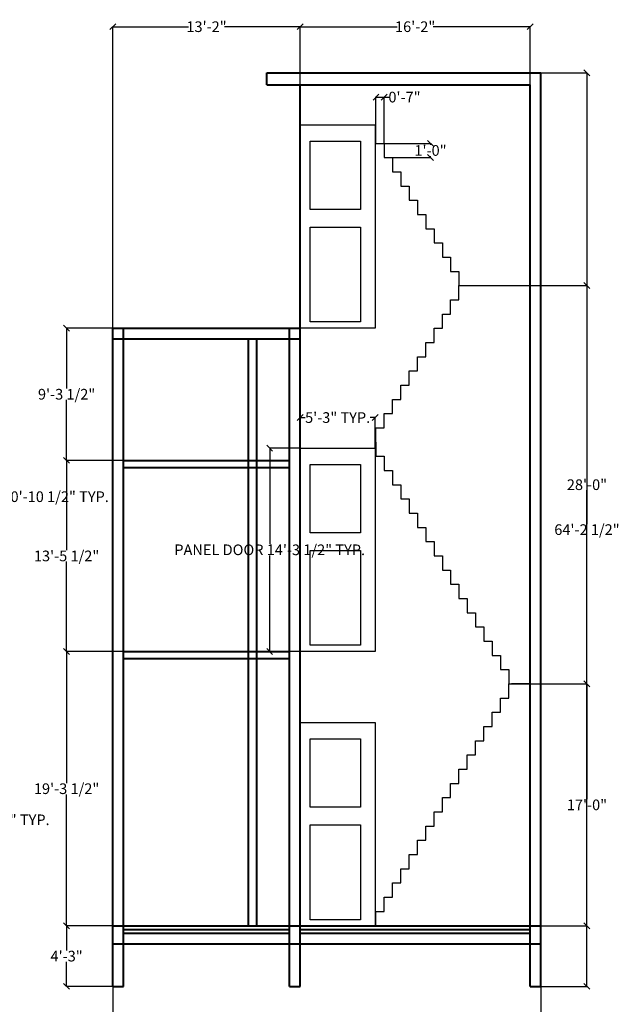
# Model space of a CAD drawing. Units: inches. Extents: x -19 to 1000, y -122 to 1144.
# Tile 8 of 8: x 486 to 991, y 313 to 1144. Entities that reach past the tile are written whole.
import ezdxf

# ---------------------------------------------------------------- set-up
doc = ezdxf.new("R2010")
doc.units = ezdxf.units.IN
doc.header["$MEASUREMENT"] = 0
for name, color, linetype, lineweight in [('A-ANNO-DIMS', 191, 'Continuous', 18), ('A-SECT', 4, 'Continuous', 40), ('A-SECT-DOOR', 2, 'Continuous', 25), ('A-SECT-STRS', 241, 'Continuous', 25)]:
    doc.layers.add(name, color=color, linetype=linetype, lineweight=lineweight)
doc.styles.get("Standard").update_dxf_attribs({"font": 'arial.ttf'})
doc.dimstyles.get("Standard").update_dxf_attribs({"dimtxt": 9, "dimasz": 5, "dimexe": 0.18, "dimexo": 0.0625, "dimgap": 0.09, "dimtad": 0, "dimtih": 1, "dimtoh": 1, "dimdec": 0, "dimzin": 0, "dimdsep": 46, "dimlunit": 3, "dimtxsty": 'Standard', "dimblk": 'OBLIQUE', "dimcen": 0.09, "dimadec": 0, "dimazin": 0, "dimtfac": 1, "dimtdec": 0, "dimtofl": 0, "dimtmove": 0, "dimatfit": 3, "dimfxl": 1, "dimtolj": 1, "dimtzin": 0, "dimarcsym": 0})

# ---------------------------------------------------------------- blocks, each defined once
blk = doc.blocks.new('DOOR-PANEL-SECTION')
for points in [[(63.17, 0), (0, 0), (0, 171.64), (63.17, 171.64)], [(50.84, 100.09), (8.47, 100.09), (8.47, 157.73), (50.84, 157.73)], [(50.84, 5.25), (8.47, 5.25), (8.47, 85.25), (50.84, 85.25)]]:
    blk.add_lwpolyline(points, close=True)
blk = doc.blocks.new('_Oblique')
at = {"color": 0, "linetype": 'ByBlock', "lineweight": -2}
blk.add_line((-0.5, -0.5), (0.5, 0.5), dxfattribs=at)
blk = doc.blocks.new('*D49')
at = {"layer": 'A-ANNO-DIMS', "color": 0, "lineweight": -2, "transparency": 16777216}
for p, q in [((722.35, 782.25), (696.49, 782.25)), ((696.67, 782.25), (696.67, 701.18)), ((696.67, 610.61), (696.67, 691.68)), ((722.35, 610.61), (696.49, 610.61))]:
    blk.add_line(p, q, dxfattribs=at)
at = {"layer": 'Defpoints', "color": 0, "transparency": 16777216}
for p in [(696.67, 782.25), (722.41, 782.25), (722.41, 610.61)]:
    blk.add_point(p, dxfattribs=at)
at = {"layer": 'A-ANNO-DIMS', "color": 0, "lineweight": -2, "transparency": 16777216, "xscale": 5, "yscale": 5, "zscale": 5}
for p, rotation in [((696.67, 782.25), 90), ((696.67, 610.61), 270)]:
    blk.add_blockref('_Oblique', p, dxfattribs=dict(at, rotation=rotation))
at = {"layer": 'A-ANNO-DIMS', "color": 0, "transparency": 16777216, "insert": (696.67, 696.43), "char_height": 9, "attachment_point": 5}
blk.add_mtext('\\A1;PANEL DOOR 14\'-3 1/2" TYP.', dxfattribs=at)
blk = doc.blocks.new('*D50')
at = {"layer": 'A-ANNO-DIMS', "color": 0, "lineweight": -2, "transparency": 16777216}
for p, q in [((722.41, 782.31), (722.41, 808.18)), ((722.41, 808), (726.48, 808)), ((785.58, 808), (781.52, 808)), ((785.58, 782.31), (785.58, 808.18))]:
    blk.add_line(p, q, dxfattribs=at)
at = {"layer": 'Defpoints', "color": 0, "transparency": 16777216}
for p in [(785.58, 808), (722.41, 782.25), (785.58, 782.25)]:
    blk.add_point(p, dxfattribs=at)
at = {"layer": 'A-ANNO-DIMS', "color": 0, "lineweight": -2, "transparency": 16777216, "xscale": 5, "yscale": 5, "zscale": 5, "rotation": 180}
blk.add_blockref('_Oblique', (722.41, 808), dxfattribs=at)
at = {"layer": 'A-ANNO-DIMS', "color": 0, "lineweight": -2, "transparency": 16777216, "xscale": 5, "yscale": 5, "zscale": 5}
blk.add_blockref('_Oblique', (785.58, 808), dxfattribs=at)
at = {"layer": 'A-ANNO-DIMS', "color": 0, "transparency": 16777216, "insert": (754, 808), "char_height": 9, "attachment_point": 5}
blk.add_mtext('\\A1;5\'-3" TYP.', dxfattribs=at)
blk = doc.blocks.new('*D73')
at = {"layer": 'A-ANNO-DIMS', "color": 0, "lineweight": -2, "transparency": 16777216}
for p, q in [((261.67, 483.28), (261.67, 468.45)), ((359.78, 483.28), (359.78, 468.45)), ((261.67, 468.63), (359.78, 468.63)), ((359.78, 468.63), (364.78, 468.63))]:
    blk.add_line(p, q, dxfattribs=at)
at = {"layer": 'Defpoints', "color": 0, "transparency": 16777216}
for p in [(261.67, 483.35), (359.78, 483.35), (359.78, 468.63)]:
    blk.add_point(p, dxfattribs=at)
at = {"layer": 'A-ANNO-DIMS', "color": 0, "lineweight": -2, "transparency": 16777216, "xscale": 5, "yscale": 5, "zscale": 5, "rotation": 180}
blk.add_blockref('_Oblique', (261.67, 468.63), dxfattribs=at)
at = {"layer": 'A-ANNO-DIMS', "color": 0, "lineweight": -2, "transparency": 16777216, "xscale": 5, "yscale": 5, "zscale": 5}
blk.add_blockref('_Oblique', (359.78, 468.63), dxfattribs=at)
at = {"layer": 'A-ANNO-DIMS', "color": 0, "transparency": 16777216, "insert": (439.97, 468.63), "char_height": 9, "attachment_point": 5}
blk.add_mtext('\\A1;WIDE WINDOW 8\'-2" TYP.', dxfattribs=at)
blk = doc.blocks.new('*D79')
at = {"layer": 'A-ANNO-DIMS', "color": 0, "lineweight": -2, "transparency": 16777216}
for p, q in [((247.56, 721.74), (247.56, 741.41)), ((247.56, 741.23), (377.88, 741.23)), ((377.88, 721.74), (377.88, 741.41)), ((377.88, 741.23), (382.88, 741.23))]:
    blk.add_line(p, q, dxfattribs=at)
at = {"layer": 'Defpoints', "color": 0, "transparency": 16777216}
for p in [(377.88, 741.23), (247.56, 721.68), (377.88, 721.68)]:
    blk.add_point(p, dxfattribs=at)
at = {"layer": 'A-ANNO-DIMS', "color": 0, "lineweight": -2, "transparency": 16777216, "xscale": 5, "yscale": 5, "zscale": 5, "rotation": 180}
blk.add_blockref('_Oblique', (247.56, 741.23), dxfattribs=at)
at = {"layer": 'A-ANNO-DIMS', "color": 0, "lineweight": -2, "transparency": 16777216, "xscale": 5, "yscale": 5, "zscale": 5}
blk.add_blockref('_Oblique', (377.88, 741.23), dxfattribs=at)
at = {"layer": 'A-ANNO-DIMS', "color": 0, "transparency": 16777216, "insert": (474.52, 741.23), "char_height": 9, "attachment_point": 5}
blk.add_mtext('\\A1;WIDE CANOPY 10\'-10 1/2" TYP.', dxfattribs=at)
blk = doc.blocks.new('*D129')
at = {"layer": 'A-ANNO-DIMS', "color": 0, "lineweight": -2, "transparency": 16777216}
for p, q in [((564.34, 328.07), (564.34, 288.95)), ((925.34, 328.07), (925.34, 288.95)), ((564.34, 289.13), (729.3, 289.13)), ((925.34, 289.13), (760.39, 289.13))]:
    blk.add_line(p, q, dxfattribs=at)
at = {"layer": 'Defpoints', "color": 0, "transparency": 16777216}
for p in [(564.34, 328.13), (925.34, 328.13), (925.34, 289.13)]:
    blk.add_point(p, dxfattribs=at)
at = {"layer": 'A-ANNO-DIMS', "color": 0, "lineweight": -2, "transparency": 16777216, "xscale": 5, "yscale": 5, "zscale": 5, "rotation": 180}
blk.add_blockref('_Oblique', (564.34, 289.13), dxfattribs=at)
at = {"layer": 'A-ANNO-DIMS', "color": 0, "lineweight": -2, "transparency": 16777216, "xscale": 5, "yscale": 5, "zscale": 5}
blk.add_blockref('_Oblique', (925.34, 289.13), dxfattribs=at)
at = {"layer": 'A-ANNO-DIMS', "color": 0, "transparency": 16777216, "insert": (744.84, 289.13), "char_height": 9, "attachment_point": 5}
blk.add_mtext('\\A1;30\'-1"', dxfattribs=at)
blk = doc.blocks.new('*D130')
at = {"layer": 'A-ANNO-DIMS', "color": 0, "lineweight": -2, "transparency": 16777216}
for p, q in [((925.41, 1098.76), (964.52, 1098.76)), ((964.34, 1098.76), (964.34, 718.19)), ((964.34, 328.13), (964.34, 708.7)), ((925.41, 328.13), (964.52, 328.13))]:
    blk.add_line(p, q, dxfattribs=at)
at = {"layer": 'Defpoints', "color": 0, "transparency": 16777216}
for p in [(925.34, 1098.76), (925.34, 328.13), (964.34, 328.13)]:
    blk.add_point(p, dxfattribs=at)
at = {"layer": 'A-ANNO-DIMS', "color": 0, "lineweight": -2, "transparency": 16777216, "xscale": 5, "yscale": 5, "zscale": 5}
for p, rotation in [((964.34, 1098.76), 90), ((964.34, 328.13), 270)]:
    blk.add_blockref('_Oblique', p, dxfattribs=dict(at, rotation=rotation))
at = {"layer": 'A-ANNO-DIMS', "color": 0, "transparency": 16777216, "insert": (964.34, 713.45), "char_height": 9, "attachment_point": 5}
blk.add_mtext('\\A1;64\'-2 1/2"', dxfattribs=at)
blk = doc.blocks.new('*D131')
at = {"layer": 'A-ANNO-DIMS', "color": 0, "lineweight": -2, "transparency": 16777216}
for p, q in [((564.34, 883.52), (564.34, 1137.94)), ((564.34, 1137.76), (628.25, 1137.76)), ((722.41, 1137.76), (658.5, 1137.76)), ((722.41, 1088.82), (722.41, 1137.94))]:
    blk.add_line(p, q, dxfattribs=at)
at = {"layer": 'Defpoints', "color": 0, "transparency": 16777216}
for p in [(722.41, 1137.76), (722.41, 1088.76), (564.34, 883.45)]:
    blk.add_point(p, dxfattribs=at)
at = {"layer": 'A-ANNO-DIMS', "color": 0, "lineweight": -2, "transparency": 16777216, "xscale": 5, "yscale": 5, "zscale": 5, "rotation": 180}
blk.add_blockref('_Oblique', (564.34, 1137.76), dxfattribs=at)
at = {"layer": 'A-ANNO-DIMS', "color": 0, "lineweight": -2, "transparency": 16777216, "xscale": 5, "yscale": 5, "zscale": 5}
blk.add_blockref('_Oblique', (722.41, 1137.76), dxfattribs=at)
at = {"layer": 'A-ANNO-DIMS', "color": 0, "transparency": 16777216, "insert": (643.38, 1137.76), "char_height": 9, "attachment_point": 5}
blk.add_mtext('\\A1;13\'-2"', dxfattribs=at)
blk = doc.blocks.new('*D132')
at = {"layer": 'A-ANNO-DIMS', "color": 0, "lineweight": -2, "transparency": 16777216}
for p, q in [((722.41, 1088.82), (722.41, 1137.94)), ((722.41, 1137.76), (804.25, 1137.76)), ((916.34, 1137.76), (834.5, 1137.76)), ((916.34, 1088.82), (916.34, 1137.94))]:
    blk.add_line(p, q, dxfattribs=at)
at = {"layer": 'Defpoints', "color": 0, "transparency": 16777216}
for p in [(916.34, 1137.76), (722.41, 1088.76), (916.34, 1088.76)]:
    blk.add_point(p, dxfattribs=at)
at = {"layer": 'A-ANNO-DIMS', "color": 0, "lineweight": -2, "transparency": 16777216, "xscale": 5, "yscale": 5, "zscale": 5, "rotation": 180}
blk.add_blockref('_Oblique', (722.41, 1137.76), dxfattribs=at)
at = {"layer": 'A-ANNO-DIMS', "color": 0, "lineweight": -2, "transparency": 16777216, "xscale": 5, "yscale": 5, "zscale": 5}
blk.add_blockref('_Oblique', (916.34, 1137.76), dxfattribs=at)
at = {"layer": 'A-ANNO-DIMS', "color": 0, "transparency": 16777216, "insert": (819.38, 1137.76), "char_height": 9, "attachment_point": 5}
blk.add_mtext('\\A1;16\'-2"', dxfattribs=at)
blk = doc.blocks.new('*D133')
at = {"layer": 'A-ANNO-DIMS', "color": 0, "lineweight": -2, "transparency": 16777216}
for p, q in [((564.28, 379.13), (525.16, 379.13)), ((525.34, 379.13), (525.34, 358.32)), ((525.34, 328.13), (525.34, 348.95)), ((564.28, 328.13), (525.16, 328.13))]:
    blk.add_line(p, q, dxfattribs=at)
at = {"layer": 'Defpoints', "color": 0, "transparency": 16777216}
for p in [(525.34, 379.13), (564.34, 379.13), (564.34, 328.13)]:
    blk.add_point(p, dxfattribs=at)
at = {"layer": 'A-ANNO-DIMS', "color": 0, "lineweight": -2, "transparency": 16777216, "xscale": 5, "yscale": 5, "zscale": 5}
for p, rotation in [((525.34, 379.13), 90), ((525.34, 328.13), 270)]:
    blk.add_blockref('_Oblique', p, dxfattribs=dict(at, rotation=rotation))
at = {"layer": 'A-ANNO-DIMS', "color": 0, "transparency": 16777216, "insert": (525.34, 353.63), "char_height": 9, "attachment_point": 5}
blk.add_mtext('\\A1;4\'-3"', dxfattribs=at)
blk = doc.blocks.new('*D134')
at = {"layer": 'A-ANNO-DIMS', "color": 0, "lineweight": -2, "transparency": 16777216}
for p, q in [((573.28, 610.6), (525.16, 610.6)), ((525.34, 610.6), (525.34, 499.61)), ((525.34, 379.13), (525.34, 490.12)), ((564.28, 379.13), (525.16, 379.13))]:
    blk.add_line(p, q, dxfattribs=at)
at = {"layer": 'Defpoints', "color": 0, "transparency": 16777216}
for p in [(525.34, 610.6), (573.34, 610.6), (564.34, 379.13)]:
    blk.add_point(p, dxfattribs=at)
at = {"layer": 'A-ANNO-DIMS', "color": 0, "lineweight": -2, "transparency": 16777216, "xscale": 5, "yscale": 5, "zscale": 5}
for p, rotation in [((525.34, 610.6), 90), ((525.34, 379.13), 270)]:
    blk.add_blockref('_Oblique', p, dxfattribs=dict(at, rotation=rotation))
at = {"layer": 'A-ANNO-DIMS', "color": 0, "transparency": 16777216, "insert": (525.34, 494.87), "char_height": 9, "attachment_point": 5}
blk.add_mtext('\\A1;19\'-3 1/2"', dxfattribs=at)
blk = doc.blocks.new('*D135')
at = {"layer": 'A-ANNO-DIMS', "color": 0, "lineweight": -2, "transparency": 16777216}
for p, q in [((573.28, 771.89), (525.16, 771.89)), ((525.34, 771.89), (525.34, 695.99)), ((525.34, 610.6), (525.34, 686.5)), ((573.28, 610.6), (525.16, 610.6))]:
    blk.add_line(p, q, dxfattribs=at)
at = {"layer": 'Defpoints', "color": 0, "transparency": 16777216}
for p in [(525.34, 771.89), (573.34, 771.89), (573.34, 610.6)]:
    blk.add_point(p, dxfattribs=at)
at = {"layer": 'A-ANNO-DIMS', "color": 0, "lineweight": -2, "transparency": 16777216, "xscale": 5, "yscale": 5, "zscale": 5}
for p, rotation in [((525.34, 771.89), 90), ((525.34, 610.6), 270)]:
    blk.add_blockref('_Oblique', p, dxfattribs=dict(at, rotation=rotation))
at = {"layer": 'A-ANNO-DIMS', "color": 0, "transparency": 16777216, "insert": (525.34, 691.25), "char_height": 9, "attachment_point": 5}
blk.add_mtext('\\A1;13\'-5 1/2"', dxfattribs=at)
blk = doc.blocks.new('*D136')
at = {"layer": 'A-ANNO-DIMS', "color": 0, "lineweight": -2, "transparency": 16777216}
for p, q in [((564.28, 883.45), (525.16, 883.45)), ((525.34, 883.45), (525.34, 832.42)), ((525.34, 771.89), (525.34, 822.93)), ((573.28, 771.89), (525.16, 771.89))]:
    blk.add_line(p, q, dxfattribs=at)
at = {"layer": 'Defpoints', "color": 0, "transparency": 16777216}
for p in [(525.34, 883.45), (564.34, 883.45), (573.34, 771.89)]:
    blk.add_point(p, dxfattribs=at)
at = {"layer": 'A-ANNO-DIMS', "color": 0, "lineweight": -2, "transparency": 16777216, "xscale": 5, "yscale": 5, "zscale": 5}
for p, rotation in [((525.34, 883.45), 90), ((525.34, 771.89), 270)]:
    blk.add_blockref('_Oblique', p, dxfattribs=dict(at, rotation=rotation))
at = {"layer": 'A-ANNO-DIMS', "color": 0, "transparency": 16777216, "insert": (525.34, 827.67), "char_height": 9, "attachment_point": 5}
blk.add_mtext('\\A1;9\'-3 1/2"', dxfattribs=at)
blk = doc.blocks.new('*D137')
at = {"layer": 'A-ANNO-DIMS', "color": 0, "lineweight": -2, "transparency": 16777216}
for p, q in [((786.34, 1039.41), (786.34, 1078.53)), ((786.34, 1078.35), (793.34, 1078.35)), ((793.34, 1039.41), (793.34, 1078.53)), ((793.34, 1078.35), (798.34, 1078.35))]:
    blk.add_line(p, q, dxfattribs=at)
at = {"layer": 'Defpoints', "color": 0, "transparency": 16777216}
for p in [(793.34, 1078.35), (786.34, 1039.35), (793.34, 1039.35)]:
    blk.add_point(p, dxfattribs=at)
at = {"layer": 'A-ANNO-DIMS', "color": 0, "lineweight": -2, "transparency": 16777216, "xscale": 5, "yscale": 5, "zscale": 5, "rotation": 180}
blk.add_blockref('_Oblique', (786.34, 1078.35), dxfattribs=at)
at = {"layer": 'A-ANNO-DIMS', "color": 0, "lineweight": -2, "transparency": 16777216, "xscale": 5, "yscale": 5, "zscale": 5}
blk.add_blockref('_Oblique', (793.34, 1078.35), dxfattribs=at)
at = {"layer": 'A-ANNO-DIMS', "color": 0, "transparency": 16777216, "insert": (810.39, 1078.35), "char_height": 9, "attachment_point": 5}
blk.add_mtext('\\A1;0\'-7"', dxfattribs=at)
blk = doc.blocks.new('*D138')
at = {"layer": 'A-ANNO-DIMS', "color": 0, "lineweight": -2, "transparency": 16777216}
for p, q in [((793.4, 1039.35), (832.52, 1039.35)), ((832.34, 1039.35), (832.34, 1038.03)), ((793.4, 1027.35), (832.52, 1027.35)), ((832.34, 1027.35), (832.34, 1028.66))]:
    blk.add_line(p, q, dxfattribs=at)
at = {"layer": 'Defpoints', "color": 0, "transparency": 16777216}
for p in [(793.34, 1039.35), (793.34, 1027.35), (832.34, 1027.35)]:
    blk.add_point(p, dxfattribs=at)
at = {"layer": 'A-ANNO-DIMS', "color": 0, "lineweight": -2, "transparency": 16777216, "xscale": 5, "yscale": 5, "zscale": 5}
for p, rotation in [((832.34, 1039.35), 90), ((832.34, 1027.35), 270)]:
    blk.add_blockref('_Oblique', p, dxfattribs=dict(at, rotation=rotation))
at = {"layer": 'A-ANNO-DIMS', "color": 0, "transparency": 16777216, "insert": (832.34, 1033.35), "char_height": 9, "attachment_point": 5}
blk.add_mtext('\\A1;1\'-0"', dxfattribs=at)
blk = doc.blocks.new('*D139')
at = {"layer": 'A-ANNO-DIMS', "color": 0, "lineweight": -2, "transparency": 16777216}
for p, q in [((916.41, 583.35), (964.52, 583.35)), ((964.34, 583.35), (964.34, 485.93)), ((964.34, 379.13), (964.34, 476.56)), ((925.41, 379.13), (964.52, 379.13))]:
    blk.add_line(p, q, dxfattribs=at)
at = {"layer": 'Defpoints', "color": 0, "transparency": 16777216}
for p in [(916.34, 583.35), (964.34, 583.35), (925.34, 379.13)]:
    blk.add_point(p, dxfattribs=at)
at = {"layer": 'A-ANNO-DIMS', "color": 0, "lineweight": -2, "transparency": 16777216, "xscale": 5, "yscale": 5, "zscale": 5}
for p, rotation in [((964.34, 583.35), 90), ((964.34, 379.13), 270)]:
    blk.add_blockref('_Oblique', p, dxfattribs=dict(at, rotation=rotation))
at = {"layer": 'A-ANNO-DIMS', "color": 0, "transparency": 16777216, "insert": (964.34, 481.24), "char_height": 9, "attachment_point": 5}
blk.add_mtext('\\A1;17\'-0"', dxfattribs=at)
blk = doc.blocks.new('*D140')
at = {"layer": 'A-ANNO-DIMS', "color": 0, "lineweight": -2, "transparency": 16777216}
for p, q in [((856.4, 919.35), (964.52, 919.35)), ((964.34, 919.35), (964.34, 756.03)), ((964.34, 583.35), (964.34, 746.66)), ((898.4, 583.35), (964.52, 583.35))]:
    blk.add_line(p, q, dxfattribs=at)
at = {"layer": 'Defpoints', "color": 0, "transparency": 16777216}
for p in [(856.34, 919.35), (964.34, 919.35), (898.34, 583.35)]:
    blk.add_point(p, dxfattribs=at)
at = {"layer": 'A-ANNO-DIMS', "color": 0, "lineweight": -2, "transparency": 16777216, "xscale": 5, "yscale": 5, "zscale": 5}
for p, rotation in [((964.34, 919.35), 90), ((964.34, 583.35), 270)]:
    blk.add_blockref('_Oblique', p, dxfattribs=dict(at, rotation=rotation))
at = {"layer": 'A-ANNO-DIMS', "color": 0, "transparency": 16777216, "insert": (964.34, 751.35), "char_height": 9, "attachment_point": 5}
blk.add_mtext('\\A1;28\'-0"', dxfattribs=at)

msp = doc.modelspace()

# ---------------------------------------------------------------- linework, layer by layer
at = {"layer": 'A-SECT'}
for p, q in [((694.18, 1098.76), (925.34, 1098.76)), ((694.18, 1088.76), (694.18, 1098.76)), ((925.34, 328.13), (925.34, 1098.76)), ((694.18, 1088.76), (916.34, 1088.76)), ((722.41, 1055.1), (722.41, 1088.76)), ((916.34, 328.13), (916.34, 1088.76)), ((722.41, 328.13), (722.41, 1055.1)), ((564.34, 797.3), (564.34, 883.45)), ((564.34, 883.45), (722.41, 883.45)), ((573.34, 797.3), (573.34, 883.45)), ((713.41, 328.13), (713.41, 883.45)), ((564.34, 874.45), (722.41, 874.45)), ((678.91, 379.13), (678.91, 874.45)), ((685.91, 379.13), (685.91, 874.45)), ((564.34, 328.13), (564.34, 797.3)), ((573.34, 328.13), (573.34, 797.3)), ((573.34, 771.89), (713.41, 771.89)), ((573.34, 765.89), (713.41, 765.89)), ((573.34, 610.6), (713.41, 610.6)), ((573.34, 604.6), (713.41, 604.6)), ((564.34, 379.13), (925.34, 379.13)), ((573.34, 376.13), (713.41, 376.13)), ((722.41, 376.13), (916.34, 376.13)), ((573.34, 373.13), (713.41, 373.13)), ((722.41, 373.13), (916.34, 373.13)), ((564.34, 364.13), (925.34, 364.13)), ((564.34, 328.13), (573.34, 328.13)), ((713.41, 328.13), (722.41, 328.13)), ((916.34, 328.13), (925.34, 328.13))]:
    msp.add_line(p, q, dxfattribs=at)
at = {"layer": 'A-SECT-STRS'}
for p, q in [((786.34, 1039.35), (793.34, 1039.35)), ((793.34, 1039.35), (793.34, 1027.35)), ((793.34, 1027.35), (800.34, 1027.35)), ((800.34, 1027.35), (800.34, 1015.35)), ((800.34, 1015.35), (807.34, 1015.35)), ((807.34, 1015.35), (807.34, 1003.35)), ((807.34, 1003.35), (814.34, 1003.35)), ((814.34, 1003.35), (814.34, 991.35)), ((814.34, 991.35), (821.34, 991.35)), ((821.34, 991.35), (821.34, 979.35)), ((821.34, 979.35), (828.34, 979.35)), ((828.34, 979.35), (828.34, 967.35)), ((828.34, 967.35), (835.34, 967.35)), ((835.34, 967.35), (835.34, 955.35)), ((835.34, 955.35), (842.34, 955.35)), ((842.34, 955.35), (842.34, 943.35)), ((842.34, 943.35), (849.34, 943.35)), ((849.34, 943.35), (849.34, 931.35)), ((849.34, 931.35), (856.34, 931.35)), ((856.34, 931.35), (856.34, 919.35)), ((856.34, 907.35), (856.34, 919.35)), ((856.34, 919.35), (863.34, 919.35)), ((849.34, 895.35), (849.34, 907.35)), ((849.34, 907.35), (856.34, 907.35)), ((842.34, 883.35), (842.34, 895.35)), ((842.34, 895.35), (849.34, 895.35)), ((835.34, 871.35), (835.34, 883.35)), ((835.34, 883.35), (842.34, 883.35)), ((828.34, 859.35), (828.34, 871.35)), ((828.34, 871.35), (835.34, 871.35)), ((821.34, 847.35), (821.34, 859.35)), ((821.34, 859.35), (828.34, 859.35)), ((814.34, 835.35), (814.34, 847.35)), ((814.34, 847.35), (821.34, 847.35)), ((807.34, 823.35), (807.34, 835.35)), ((807.34, 835.35), (814.34, 835.35)), ((800.34, 811.35), (800.34, 823.35)), ((800.34, 823.35), (807.34, 823.35)), ((793.34, 799.35), (793.34, 811.35)), ((793.34, 811.35), (800.34, 811.35)), ((786.34, 787.35), (786.34, 799.35)), ((786.34, 799.35), (793.34, 799.35)), ((786.34, 787.35), (786.34, 775.35)), ((786.34, 775.35), (793.34, 775.35)), ((793.34, 775.35), (793.34, 763.35)), ((793.34, 763.35), (800.34, 763.35)), ((800.34, 763.35), (800.34, 751.35)), ((800.34, 751.35), (807.34, 751.35)), ((807.34, 751.35), (807.34, 739.35)), ((807.34, 739.35), (814.34, 739.35)), ((814.34, 739.35), (814.34, 727.35)), ((814.34, 727.35), (821.34, 727.35)), ((821.34, 727.35), (821.34, 715.35)), ((821.34, 715.35), (828.34, 715.35)), ((828.34, 715.35), (828.34, 703.35)), ((828.34, 703.35), (835.34, 703.35)), ((835.34, 703.35), (835.34, 691.35)), ((835.34, 691.35), (842.34, 691.35)), ((842.34, 691.35), (842.34, 679.35)), ((842.34, 679.35), (849.34, 679.35)), ((849.34, 679.35), (849.34, 667.35)), ((849.34, 667.35), (856.34, 667.35)), ((856.34, 667.35), (856.34, 655.35)), ((856.34, 655.35), (863.34, 655.35)), ((863.34, 655.35), (863.34, 643.35)), ((863.34, 643.35), (870.34, 643.35)), ((870.34, 643.35), (870.34, 631.35)), ((870.34, 631.35), (877.34, 631.35)), ((877.34, 631.35), (877.34, 619.35)), ((877.34, 619.35), (884.34, 619.35)), ((884.34, 619.35), (884.34, 607.35)), ((884.34, 607.35), (891.34, 607.35)), ((891.34, 607.35), (891.34, 595.35)), ((891.34, 595.35), (898.34, 595.35)), ((898.34, 595.35), (898.34, 583.35)), ((898.34, 571.35), (898.34, 583.35)), ((898.34, 583.35), (905.34, 583.35)), ((898.34, 583.35), (905.34, 583.35)), ((916.34, 583.35), (900.59, 583.35)), ((891.34, 559.35), (891.34, 571.35)), ((891.34, 571.35), (898.34, 571.35)), ((884.34, 547.35), (884.34, 559.35)), ((884.34, 559.35), (891.34, 559.35)), ((877.34, 535.35), (877.34, 547.35)), ((877.34, 547.35), (884.34, 547.35)), ((870.34, 523.35), (870.34, 535.35)), ((870.34, 535.35), (877.34, 535.35)), ((863.34, 511.35), (863.34, 523.35)), ((863.34, 523.35), (870.34, 523.35)), ((856.34, 499.35), (856.34, 511.35)), ((856.34, 511.35), (863.34, 511.35)), ((849.34, 487.35), (849.34, 499.35)), ((849.34, 499.35), (856.34, 499.35)), ((842.34, 475.35), (842.34, 487.35)), ((842.34, 487.35), (849.34, 487.35)), ((835.34, 463.35), (835.34, 475.35)), ((835.34, 475.35), (842.34, 475.35)), ((828.34, 451.35), (828.34, 463.35)), ((828.34, 463.35), (835.34, 463.35)), ((821.34, 439.35), (821.34, 451.35)), ((821.34, 451.35), (828.34, 451.35)), ((814.34, 427.35), (814.34, 439.35)), ((814.34, 439.35), (821.34, 439.35)), ((807.34, 415.35), (807.34, 427.35)), ((807.34, 427.35), (814.34, 427.35)), ((800.34, 403.35), (800.34, 415.35)), ((800.34, 415.35), (807.34, 415.35)), ((793.34, 391.35), (793.34, 403.35)), ((793.34, 403.35), (800.34, 403.35)), ((786.34, 379.35), (786.34, 391.35)), ((786.34, 391.35), (793.34, 391.35))]:
    msp.add_line(p, q, dxfattribs=at)

# ---------------------------------------------------------------- block references
at = {"layer": 'A-SECT-DOOR'}
for p in [(722.41, 883.45), (722.41, 610.61), (722.41, 379.13)]:
    msp.add_blockref('DOOR-PANEL-SECTION', p, dxfattribs=at)

# ---------------------------------------------------------------- dimensions: what is measured, and where the dimension line sits
at = {"layer": 'A-ANNO-DIMS'}
for base, p1, p2, picture, middle in [((722.41, 1137.76), (564.34, 883.45), (722.41, 1088.76), '*D131', (643.38, 1137.76)), ((916.34, 1137.76), (722.41, 1088.76), (916.34, 1088.76), '*D132', (819.38, 1137.76)), ((793.34, 1078.35), (786.34, 1039.35), (793.34, 1039.35), '*D137', (810.39, 1078.35)), ((925.34, 289.13), (564.34, 328.13), (925.34, 328.13), '*D129', (744.84, 289.13))]:
    dim = msp.add_linear_dim(base=base, p1=p1, p2=p2, dimstyle='Standard', override={"dimdec": 1, "dimlfac": 1, "dimrnd": 0, "dimzin": 1, "dimdsep": 46, "dimlunit": 4, "dimfrac": 2}, dxfattribs=at)
    dim.commit()
    dim.dimension.update_dxf_attribs({"geometry": picture, "text_midpoint": middle})
for base, p1, p2, angle, picture, middle in [((964.34, 328.13), (925.34, 1098.76), (925.34, 328.13), 270, '*D130', (964.34, 713.45)), ((832.34, 1027.35), (793.34, 1039.35), (793.34, 1027.35), 270, '*D138', (832.34, 1033.35)), ((964.34, 919.35), (898.34, 583.35), (856.34, 919.35), 90, '*D140', (964.34, 751.35)), ((525.34, 883.45), (573.34, 771.89), (564.34, 883.45), 90, '*D136', (525.34, 827.67)), ((525.34, 771.89), (573.34, 610.6), (573.34, 771.89), 90, '*D135', (525.34, 691.25)), ((525.34, 610.6), (564.34, 379.13), (573.34, 610.6), 90, '*D134', (525.34, 494.87)), ((964.34, 583.35), (925.34, 379.13), (916.34, 583.35), 90, '*D139', (964.34, 481.24)), ((525.34, 379.13), (564.34, 328.13), (564.34, 379.13), 90, '*D133', (525.34, 353.63))]:
    dim = msp.add_linear_dim(base=base, p1=p1, p2=p2, angle=angle, dimstyle='Standard', override={"dimdec": 1, "dimlfac": 1, "dimrnd": 0, "dimzin": 1, "dimdsep": 46, "dimlunit": 4, "dimfrac": 2}, dxfattribs=at)
    dim.commit()
    dim.dimension.update_dxf_attribs({"geometry": picture, "text_midpoint": middle})
for base, p1, p2, text, picture, middle in [((785.58, 808), (722.41, 782.25), (785.58, 782.25), '<> TYP.', '*D50', (754, 808)), ((377.88, 741.23), (247.56, 721.68), (377.88, 721.68), 'WIDE CANOPY <> TYP.', '*D79', (474.52, 741.23)), ((359.78, 468.63), (261.67, 483.35), (359.78, 483.35), 'WIDE WINDOW <> TYP.', '*D73', (439.97, 468.63))]:
    dim = msp.add_linear_dim(base=base, p1=p1, p2=p2, text=text, dimstyle='Standard', override={"dimdec": 1, "dimlfac": 1, "dimrnd": 0, "dimzin": 1, "dimdsep": 46, "dimlunit": 4, "dimfrac": 2}, dxfattribs=at)
    dim.commit()
    dim.dimension.update_dxf_attribs({"geometry": picture, "text_midpoint": middle})
dim = msp.add_linear_dim(base=(696.67, 782.25), p1=(722.41, 610.61), p2=(722.41, 782.25), angle=90, text='PANEL DOOR <> TYP.', dimstyle='Standard', override={"dimdec": 1, "dimlfac": 1, "dimrnd": 0, "dimzin": 1, "dimdsep": 46, "dimlunit": 4, "dimfrac": 2}, dxfattribs=at)
dim.commit()
dim.dimension.update_dxf_attribs({"geometry": '*D49', "text_midpoint": (696.67, 696.43)})

doc.saveas('drawing.dxf')
